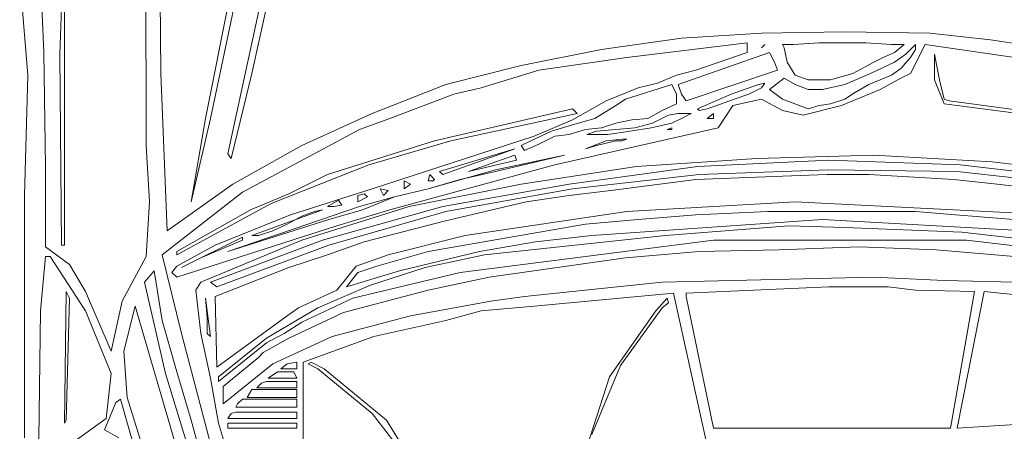
# Model space of a CAD drawing. Units: inches. Extents: x -36302355 to 648, y -221479757 to 75.
# Tile 8 of 37: x 185 to 209, y -465 to -455. Entities that reach past the tile are written whole.
import ezdxf

# ---------------------------------------------------------------- set-up
doc = ezdxf.new("R2010")
doc.units = ezdxf.units.IN
doc.header["$MEASUREMENT"] = 0
doc.layers.add('A-EQPM-VEHC', color=8, linetype='Continuous', lineweight=13)

msp = doc.modelspace()

# ---------------------------------------------------------------- linework, layer by layer
at = {"layer": 'A-EQPM-VEHC'}
for p, q in [((190.101, -458.196), (193.287, -443.449)), ((193.326, -444.079), (190.69, -456.23)), ((188.37, -444.944), (188.449, -456.23)), ((192.068, -446.045), (189.669, -457.331)), ((186.326, -446.517), (185.972, -455.758)), ((188.095, -457.369), (188.056, -448.287)), ((189.551, -457.331), (190.927, -450.41)), ((185.5, -453.753), (185.579, -455.718)), ((184.989, -453.87), (185.186, -456.269)), ((186.089, -460.437), (186.089, -454.618)), ((201.229, -455.365), (203.196, -455.246)), ((203.196, -455.246), (205.24, -455.207)), ((205.24, -455.207), (207.325, -455.246)), ((207.325, -455.246), (208.818, -455.404)), ((199.264, -455.639), (201.229, -455.365)), ((202.841, -455.483), (199.892, -455.836)), ((202.841, -455.718), (202.841, -455.483)), ((204.612, -455.483), (203.982, -455.522)), ((205.751, -455.483), (204.612, -455.483)), ((206.381, -455.522), (205.751, -455.483)), ((208.818, -455.404), (210.313, -455.639)), ((185.579, -455.718), (185.619, -458.51)), ((197.297, -456.034), (199.264, -455.639)), ((203.392, -455.718), (201.152, -456.504)), ((201.583, -456.151), (202.841, -455.718)), ((203.196, -455.601), (203.275, -455.522)), ((203.51, -455.955), (203.392, -455.718)), ((203.982, -455.522), (203.707, -455.522)), ((203.707, -455.522), (203.747, -455.601)), ((203.747, -455.601), (203.824, -455.955)), ((206.184, -455.836), (206.46, -455.718)), ((206.695, -455.522), (206.381, -455.522)), ((206.46, -455.718), (206.695, -455.522)), ((206.97, -455.522), (206.735, -455.758)), ((207.207, -455.522), (206.853, -456.23)), ((206.853, -455.836), (206.97, -455.639)), ((206.97, -455.639), (206.97, -455.522)), ((210.195, -455.955), (207.207, -455.522)), ((185.972, -455.758), (186.012, -460.437)), ((199.892, -455.836), (197.73, -456.151)), ((203.589, -456.151), (203.51, -455.955)), ((203.824, -455.955), (204.021, -456.269)), ((205.437, -456.23), (205.949, -455.955)), ((206.46, -455.955), (205.87, -456.23)), ((205.949, -455.955), (206.184, -455.836)), ((206.735, -455.758), (206.46, -455.955)), ((206.616, -456.111), (206.853, -455.836)), ((207.56, -456.387), (207.442, -455.758)), ((207.442, -455.758), (207.442, -456.387)), ((195.449, -456.504), (197.297, -456.034)), ((197.73, -456.151), (196.314, -456.583)), ((201.111, -456.269), (201.583, -456.151)), ((201.348, -456.899), (203.589, -456.151)), ((206.381, -456.269), (206.616, -456.111)), ((185.186, -456.269), (185.107, -459.219)), ((188.449, -456.23), (188.607, -460.084)), ((190.69, -456.23), (190.18, -458.313)), ((200.639, -456.466), (201.111, -456.269)), ((203.747, -456.348), (203.392, -456.623)), ((204.021, -456.504), (203.747, -456.348)), ((204.021, -456.269), (204.336, -456.387)), ((204.336, -456.387), (204.886, -456.387)), ((204.886, -456.387), (205.437, -456.23)), ((205.87, -456.23), (205.24, -456.504)), ((205.83, -456.504), (206.381, -456.269)), ((206.616, -456.348), (206.105, -456.623)), ((206.853, -456.23), (206.616, -456.348)), ((207.442, -456.387), (207.679, -456.976)), ((207.679, -456.859), (207.56, -456.387)), ((193.64, -457.213), (195.449, -456.504)), ((196.314, -456.583), (195.645, -456.741)), ((199.381, -456.899), (200.167, -456.583)), ((200.994, -456.504), (199.853, -456.859)), ((200.167, -456.583), (200.639, -456.466)), ((201.111, -456.741), (200.994, -456.504)), ((201.152, -456.504), (201.229, -456.741)), ((203.117, -456.504), (202.448, -456.741)), ((202.882, -456.741), (203.196, -456.583)), ((203.275, -456.466), (203.117, -456.504)), ((203.196, -456.583), (203.275, -456.466)), ((203.392, -456.623), (203.707, -456.859)), ((204.336, -456.623), (204.021, -456.504)), ((204.689, -456.623), (204.336, -456.623)), ((205.24, -456.504), (204.689, -456.623)), ((206.105, -456.623), (205.161, -457.017)), ((205.477, -456.701), (205.83, -456.504)), ((195.645, -456.741), (194.073, -457.331)), ((198.555, -457.369), (199.381, -456.899)), ((199.853, -456.859), (199.618, -457.017)), ((201.111, -456.976), (201.111, -456.741)), ((201.229, -456.741), (201.348, -456.899)), ((202.448, -456.741), (201.622, -457.095)), ((202.213, -456.976), (202.527, -456.859)), ((203.196, -456.859), (202.487, -457.017)), ((202.527, -456.859), (202.882, -456.741)), ((203.707, -457.134), (203.196, -456.859)), ((203.707, -456.859), (204.336, -457.095)), ((204.886, -456.976), (205.24, -456.859)), ((205.24, -456.859), (205.477, -456.701)), ((207.797, -456.899), (207.679, -456.859)), ((211.296, -457.369), (207.797, -456.899)), ((198.555, -457.095), (195.173, -457.882)), ((198.674, -457.213), (198.555, -457.095)), ((199.618, -457.017), (199.106, -457.331)), ((200.404, -457.331), (200.757, -457.134)), ((200.757, -457.134), (201.111, -456.976)), ((201.622, -457.095), (201.662, -457.134)), ((201.662, -457.134), (201.859, -457.095)), ((201.859, -457.095), (202.213, -456.976)), ((202.487, -457.017), (202.134, -457.566)), ((204.217, -457.252), (203.707, -457.134)), ((205.161, -457.017), (204.217, -457.252)), ((204.336, -457.095), (204.612, -457.017)), ((204.612, -457.017), (204.886, -456.976)), ((207.679, -456.976), (211.336, -457.448)), ((188.095, -457.999), (188.095, -457.369)), ((189.669, -457.331), (189.197, -459.375)), ((189.197, -459.375), (189.551, -457.331)), ((191.91, -457.999), (193.64, -457.213)), ((194.073, -457.331), (193.326, -457.606)), ((195.567, -457.882), (198.674, -457.213)), ((197.612, -457.764), (198.555, -457.369)), ((199.106, -457.331), (198.555, -457.489)), ((199.618, -457.448), (200.011, -457.369)), ((200.011, -457.369), (200.404, -457.331)), ((200.915, -457.252), (200.522, -457.448)), ((201.152, -457.213), (200.915, -457.252)), ((200.994, -457.448), (201.229, -457.331)), ((201.466, -457.213), (201.152, -457.213)), ((201.229, -457.331), (201.466, -457.213)), ((202.017, -457.213), (201.859, -457.331)), ((201.859, -457.331), (202.017, -457.331)), ((202.017, -457.331), (202.017, -457.213)), ((193.326, -457.606), (192.657, -457.961)), ((198.044, -457.645), (197.533, -457.882)), ((198.555, -457.489), (198.044, -457.645)), ((202.134, -457.566), (198.123, -458.471)), ((198.477, -457.724), (198.871, -457.606)), ((198.871, -457.606), (199.264, -457.566)), ((199.146, -457.645), (198.909, -457.724)), ((199.618, -457.606), (199.146, -457.645)), ((199.264, -457.566), (199.618, -457.448)), ((199.42, -457.724), (199.971, -457.645)), ((200.088, -457.566), (199.618, -457.606)), ((199.971, -457.645), (200.483, -457.566)), ((200.522, -457.448), (200.088, -457.566)), ((200.483, -457.566), (200.994, -457.448)), ((200.994, -457.566), (200.876, -457.606)), ((200.876, -457.606), (200.994, -457.606)), ((200.994, -457.606), (200.994, -457.566)), ((195.173, -457.882), (192.54, -458.706)), ((193.561, -458.471), (195.567, -457.882)), ((193.64, -459.061), (197.612, -457.764)), ((197.533, -457.882), (197.297, -457.999)), ((197.73, -457.961), (198.123, -457.764)), ((198.123, -457.764), (198.477, -457.724)), ((199.381, -457.882), (198.871, -458.078)), ((198.909, -457.724), (199.42, -457.724)), ((199.146, -457.999), (199.618, -457.882)), ((199.774, -457.841), (199.381, -457.882)), ((199.618, -457.882), (199.774, -457.882)), ((199.774, -457.882), (199.892, -457.841)), ((199.892, -457.841), (199.774, -457.841)), ((188.174, -459.375), (188.095, -457.999)), ((190.22, -458.943), (191.91, -457.999)), ((192.657, -457.961), (190.455, -459.14)), ((197.14, -458.078), (195.291, -458.629)), ((195.37, -458.706), (197.14, -458.078)), ((197.297, -457.999), (197.376, -458.117)), ((197.376, -458.117), (197.73, -457.961)), ((198.871, -458.078), (199.146, -457.999)), ((190.18, -458.313), (190.101, -458.196)), ((197.14, -458.234), (196, -458.629)), ((196, -458.629), (197.179, -458.354)), ((196.668, -458.589), (198.358, -458.234)), ((198.358, -458.234), (196.668, -458.629)), ((197.179, -458.354), (197.14, -458.234)), ((203.078, -458.313), (200.129, -458.51)), ((204.847, -458.354), (201.622, -458.51)), ((205.949, -458.234), (203.078, -458.313)), ((208.072, -458.471), (204.847, -458.354)), ((208.858, -458.392), (205.949, -458.234)), ((185.619, -458.51), (185.619, -460.477)), ((191.162, -459.415), (193.561, -458.471)), ((198.123, -458.471), (194.073, -459.572)), ((195.017, -459.061), (196.668, -458.589)), ((195.291, -458.629), (195.37, -458.706)), ((196.668, -458.629), (195.803, -458.826)), ((200.129, -458.51), (197.297, -458.943)), ((201.622, -458.51), (198.477, -458.943)), ((201.662, -458.706), (204.847, -458.589)), ((204.847, -458.589), (207.993, -458.629)), ((207.993, -458.629), (211.099, -458.982)), ((211.217, -458.826), (208.072, -458.471)), ((211.689, -458.747), (208.858, -458.392)), ((192.54, -458.706), (191.596, -459.178)), ((194.426, -458.864), (194.426, -459.061)), ((194.584, -458.943), (194.426, -458.864)), ((195.056, -458.706), (195.017, -458.864)), ((195.803, -458.826), (195.017, -459.061)), ((195.017, -458.864), (195.135, -458.864)), ((195.173, -458.826), (195.056, -458.706)), ((195.135, -458.864), (195.173, -458.826)), ((198.555, -459.061), (201.662, -458.706)), ((201.583, -458.826), (199.499, -459.1)), ((203.707, -458.747), (201.583, -458.826)), ((204.808, -458.706), (203.707, -458.747)), ((205.83, -458.706), (204.808, -458.706)), ((207.914, -458.826), (205.83, -458.706)), ((208.976, -458.943), (207.914, -458.826)), ((188.607, -460.084), (190.22, -458.943)), ((191.634, -459.691), (193.64, -459.061)), ((194.033, -459.1), (193.836, -459.061)), ((193.836, -459.061), (193.915, -459.219)), ((193.915, -459.219), (194.033, -459.1)), ((195.017, -459.061), (194.191, -459.257)), ((194.426, -459.061), (194.584, -458.943)), ((197.297, -458.943), (194.545, -459.494)), ((198.477, -458.943), (195.37, -459.494)), ((195.449, -459.612), (198.555, -459.061)), ((199.499, -459.1), (198.477, -459.219)), ((211.06, -459.178), (208.976, -458.943)), ((185.107, -459.219), (185.107, -465.157)), ((190.455, -459.14), (188.488, -460.673)), ((191.596, -459.178), (190.652, -459.572)), ((192.815, -459.336), (192.54, -459.494)), ((192.892, -459.454), (192.815, -459.336)), ((193.443, -459.178), (193.287, -459.219)), ((193.287, -459.219), (193.287, -459.375)), ((193.287, -459.375), (193.522, -459.257)), ((194.191, -459.257), (193.326, -459.494)), ((193.405, -459.572), (194.191, -459.257)), ((193.522, -459.257), (193.443, -459.178)), ((198.477, -459.219), (197.416, -459.375)), ((188.095, -460.712), (188.174, -459.375)), ((188.842, -460.673), (191.162, -459.415)), ((190.652, -459.572), (188.842, -460.594)), ((193.326, -459.494), (190.101, -460.594)), ((192.42, -459.572), (190.69, -460.201)), ((194.545, -459.494), (191.91, -460.319)), ((192.224, -459.612), (192.42, -459.572)), ((195.37, -459.494), (192.42, -460.319)), ((192.54, -459.494), (192.696, -459.494)), ((192.578, -459.808), (193.405, -459.572)), ((192.696, -459.494), (192.892, -459.454)), ((194.073, -459.572), (192.775, -459.966)), ((197.416, -459.375), (195.41, -459.847)), ((199.892, -459.612), (204.021, -459.375)), ((204.021, -459.375), (210.274, -459.691)), ((189.786, -460.437), (191.634, -459.691)), ((190.101, -460.594), (192.578, -459.808)), ((191.555, -459.926), (191.91, -459.729)), ((191.91, -459.729), (192.224, -459.612)), ((192.578, -460.437), (195.449, -459.612)), ((195.921, -460.201), (199.892, -459.612)), ((200.167, -459.808), (198.871, -459.926)), ((199.027, -460.201), (204.689, -459.808)), ((201.583, -459.691), (200.167, -459.808)), ((203.352, -459.612), (201.583, -459.691)), ((206.97, -459.612), (203.352, -459.612)), ((204.689, -459.808), (210.313, -460.122)), ((207.953, -459.691), (206.97, -459.612)), ((209.841, -459.847), (207.953, -459.691)), ((192.775, -459.966), (188.842, -461.224)), ((191.202, -460.084), (191.555, -459.926)), ((195.41, -459.847), (193.443, -460.359)), ((198.871, -459.926), (195.017, -460.594)), ((203.864, -459.966), (200.836, -460.201)), ((205.24, -460.005), (203.864, -459.966)), ((208.111, -460.122), (205.24, -460.005)), ((190.455, -460.24), (188.96, -460.988)), ((191.91, -460.319), (189.432, -461.342)), ((189.432, -460.752), (190.455, -460.319)), ((192.42, -460.319), (189.669, -461.342)), ((190.455, -460.319), (190.455, -460.24)), ((190.69, -460.201), (190.848, -460.201)), ((190.848, -460.201), (191.202, -460.084)), ((194.033, -460.673), (195.921, -460.201)), ((195.803, -461.105), (202.017, -460.319)), ((200.836, -460.201), (196.393, -460.673)), ((197.651, -460.359), (199.027, -460.201)), ((202.017, -460.319), (208.228, -460.319)), ((213.263, -460.712), (208.111, -460.122)), ((208.228, -460.319), (212.633, -460.831)), ((185.619, -460.477), (186.209, -460.909)), ((186.012, -460.437), (186.089, -460.437)), ((188.842, -460.949), (189.786, -460.437)), ((189.825, -461.46), (192.578, -460.437)), ((193.443, -460.359), (192.54, -460.673)), ((196.275, -460.594), (197.651, -460.359)), ((203.628, -460.556), (201.662, -460.594)), ((205.595, -460.477), (203.628, -460.556)), ((207.483, -460.556), (205.595, -460.477)), ((211.296, -460.87), (207.483, -460.556)), ((185.5, -462.049), (185.619, -460.712)), ((185.619, -460.712), (185.737, -460.712)), ((185.737, -460.712), (186.602, -462.049)), ((187.505, -461.814), (188.095, -460.712)), ((188.488, -460.673), (188.96, -462.6)), ((188.842, -460.594), (188.842, -460.673)), ((188.96, -460.988), (189.432, -460.752)), ((192.54, -460.673), (191.596, -460.988)), ((193.247, -460.949), (194.033, -460.673)), ((195.017, -460.594), (193.757, -460.949)), ((194.308, -461.066), (196.275, -460.594)), ((196.393, -460.673), (194.938, -460.988)), ((199.853, -460.752), (196.511, -461.224)), ((201.662, -460.594), (199.853, -460.752)), ((186.209, -460.909), (186.602, -461.577)), ((188.725, -461.105), (188.842, -460.949)), ((191.596, -460.988), (189.786, -461.696)), ((192.775, -461.538), (193.247, -460.949)), ((193.757, -460.949), (193.287, -461.105)), ((194.938, -460.988), (193.601, -461.421)), ((188.292, -461.066), (188.056, -461.342)), ((188.488, -462.286), (188.292, -461.066)), ((188.842, -461.224), (188.725, -461.105)), ((193.012, -461.46), (194.308, -461.066)), ((193.287, -461.105), (193.012, -461.46)), ((193.168, -461.735), (195.803, -461.105)), ((196.511, -461.224), (195.017, -461.538)), ((200.757, -461.342), (205.949, -461.224)), ((205.949, -461.224), (207.679, -461.302)), ((188.056, -461.342), (188.567, -463.583)), ((189.432, -461.342), (189.314, -461.538)), ((189.669, -461.342), (189.825, -461.46)), ((193.601, -461.421), (192.303, -461.97)), ((197.376, -461.696), (200.757, -461.342)), ((204.847, -461.46), (201.348, -461.617)), ((206.302, -461.46), (204.847, -461.46)), ((206.97, -461.538), (206.302, -461.46)), ((207.679, -461.302), (209.409, -461.342)), ((186.089, -464.802), (186.13, -461.577)), ((186.13, -461.577), (186.209, -461.735)), ((186.209, -461.735), (186.13, -464.723)), ((186.602, -461.577), (187.23, -463.032)), ((189.314, -461.538), (189.432, -462.6)), ((189.551, -461.735), (189.669, -462.679)), ((189.59, -462.207), (189.551, -461.735)), ((189.786, -461.696), (189.825, -463.426)), ((191.831, -461.97), (192.775, -461.538)), ((191.91, -462.325), (193.168, -461.735)), ((195.017, -461.538), (192.933, -462.089)), ((196.551, -461.814), (197.376, -461.696)), ((201.032, -461.617), (197.612, -461.932)), ((200.601, -462.049), (200.876, -461.735)), ((200.876, -461.735), (200.915, -461.853)), ((202.134, -466.571), (201.032, -461.617)), ((201.348, -461.617), (201.348, -461.696)), ((201.348, -461.696), (202.017, -464.92)), ((208.425, -461.577), (206.97, -461.538)), ((207.835, -464.92), (208.425, -461.577)), ((208.662, -461.577), (207.993, -464.92)), ((213.222, -462.049), (208.662, -461.577)), ((187.23, -463.032), (187.505, -461.814)), ((187.821, -461.932), (187.546, -463.032)), ((188.842, -465.431), (187.821, -461.932)), ((192.303, -461.97), (191.045, -462.718)), ((191.555, -462.167), (191.831, -461.97)), ((194.584, -462.167), (196.551, -461.814)), ((197.612, -461.932), (196.314, -462.049)), ((200.757, -461.97), (199.736, -463.386)), ((200.915, -461.853), (200.757, -461.97)), ((185.461, -465.195), (185.5, -462.049)), ((186.602, -462.049), (187.23, -463.583)), ((189.59, -462.6), (189.59, -462.207)), ((189.825, -463.426), (191.555, -462.167)), ((192.933, -462.089), (191.596, -462.718)), ((192.657, -462.679), (194.584, -462.167)), ((196.314, -462.049), (195.449, -462.286)), ((199.46, -463.662), (200.601, -462.049)), ((188.842, -463.544), (188.488, -462.286)), ((191.478, -462.6), (191.91, -462.325)), ((195.449, -462.286), (193.68, -462.679)), ((188.96, -462.6), (189.708, -465.431)), ((189.432, -462.6), (189.669, -463.7)), ((189.669, -462.679), (189.59, -462.6)), ((191.045, -462.718), (189.865, -463.662)), ((191.596, -462.718), (190.966, -463.072)), ((191.045, -462.835), (191.478, -462.6)), ((191.202, -463.348), (192.657, -462.679)), ((193.68, -462.679), (191.95, -463.307)), ((189.865, -463.779), (191.045, -462.835)), ((187.546, -463.032), (187.623, -464.172)), ((190.848, -463.19), (189.983, -463.898)), ((190.966, -463.072), (190.848, -463.19)), ((189.983, -464.33), (191.202, -463.348)), ((191.399, -463.465), (191.555, -463.348)), ((191.792, -463.465), (191.399, -463.465)), ((191.555, -463.348), (191.792, -463.307)), ((191.792, -463.307), (191.792, -463.465)), ((191.95, -463.307), (191.95, -465.588)), ((192.146, -463.307), (192.068, -463.348)), ((192.068, -463.348), (192.303, -463.465)), ((192.461, -463.465), (192.146, -463.307)), ((192.303, -463.465), (193.64, -464.565)), ((193.994, -464.723), (192.461, -463.465)), ((199.736, -463.386), (199.027, -465.078)), ((187.23, -463.583), (187.112, -464.685)), ((188.567, -463.583), (189.786, -467.555)), ((189.197, -464.723), (188.842, -463.544)), ((189.669, -463.7), (189.865, -464.802)), ((189.865, -463.662), (189.865, -463.779)), ((191.085, -463.7), (191.32, -463.544)), ((191.792, -463.7), (191.085, -463.7)), ((191.32, -463.544), (191.713, -463.544)), ((191.713, -463.544), (191.792, -463.7)), ((198.909, -465.392), (199.46, -463.662)), ((189.983, -463.898), (189.983, -464.33)), ((190.809, -463.937), (190.927, -463.82)), ((191.792, -463.937), (190.809, -463.937)), ((190.927, -463.82), (191.045, -463.779)), ((191.045, -463.779), (191.792, -463.779)), ((191.792, -463.779), (191.792, -463.937)), ((187.623, -464.172), (188.095, -465.667)), ((190.573, -464.172), (190.69, -463.976)), ((191.792, -464.172), (190.573, -464.172)), ((190.69, -463.976), (191.792, -463.976)), ((191.792, -463.976), (191.792, -464.172)), ((187.074, -464.96), (187.349, -464.292)), ((187.349, -464.292), (187.467, -464.213)), ((187.467, -464.213), (188.095, -466.415)), ((190.297, -464.409), (190.337, -464.33)), ((191.792, -464.409), (190.297, -464.409)), ((190.337, -464.33), (190.455, -464.213)), ((190.455, -464.213), (191.792, -464.213)), ((191.792, -464.213), (191.792, -464.409)), ((190.101, -464.685), (190.18, -464.565)), ((190.18, -464.565), (190.297, -464.527)), ((190.297, -464.527), (191.792, -464.527)), ((191.792, -464.527), (191.792, -464.685)), ((193.64, -464.565), (194.78, -466.022)), ((186.13, -464.723), (186.089, -464.802)), ((187.112, -464.685), (186.405, -465.195)), ((189.865, -467.162), (189.197, -464.723)), ((189.865, -464.802), (190.18, -465.825)), ((191.792, -464.685), (190.101, -464.685)), ((190.101, -464.92), (190.101, -464.802)), ((190.101, -464.802), (191.792, -464.802)), ((191.792, -464.802), (191.792, -464.92)), ((194.938, -466.257), (193.994, -464.723)), ((207.993, -464.92), (209.959, -464.802)), ((187.426, -465.157), (187.074, -464.96)), ((191.792, -464.92), (190.101, -464.92)), ((202.017, -464.92), (207.835, -464.92))]:
    msp.add_line(p, q, dxfattribs=at)

doc.saveas('drawing.dxf')
